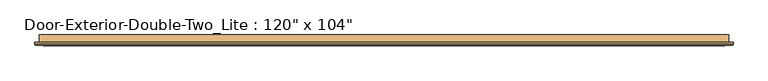
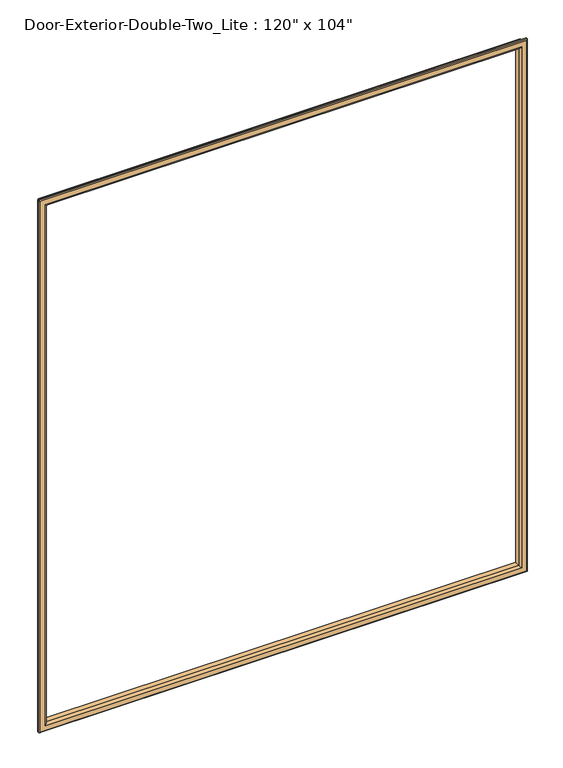
"""IFC4 building model written with IfcOpenShell, lengths in millimetres: door geometry."""

from ifc_helpers import new_model, si_unit, frame, origin, place, context, project, spatial, ellipse_curve, source, transform, mapped, element, save
from ifc_brep_helpers import plane_surface, cylinder_surface, advanced_brep


def door_2971dfc0(model_context):
    return source(origin(), model_context, "Body", "AdvancedBrep", [
        advanced_brep(
        [(-1371.6, 50.8, 1117.6), (-1371.6, 38.1, 1117.6), (-1371.6, 38.1, 2524.125), (-1371.6, 50.8, 2524.125), (-1359.6, 37.1, 1129.6), (-1359.6, 50.8, 1129.6), (-1359.6, 50.8, 2512.125), (-1359.6, 37.1, 2512.125), (-1364.6, 32.1, 1124.6), (-1364.6, 32.1, 2517.125), (-1379.6, 34.1, 1109.6), (-1377.6, 32.1, 1111.6), (-1377.6, 32.1, 2530.125), (-1379.6, 34.1, 2532.125), (-1379.6, 38.1, 1109.6), (-1379.6, 38.1, 2532.125), (-152.4, 38.1, 2524.125), (-152.4, 50.8, 2524.125), (-164.4, 50.8, 2512.125), (-164.4, 37.1, 2512.125), (-159.4, 32.1, 2517.125), (-146.4, 32.1, 2530.125), (-144.4, 34.1, 2532.125), (-144.4, 38.1, 2532.125), (-152.4, 38.1, 1117.6), (-152.4, 50.8, 1117.6), (-164.4, 50.8, 1129.6), (-164.4, 37.1, 1129.6), (-159.4, 32.1, 1124.6), (-146.4, 32.1, 1111.6), (-144.4, 34.1, 1109.6), (-144.4, 38.1, 1109.6)],
        [
            (0, 1),
            (1, 2),
            (2, 3),
            (3, 0),
            (4, 5),
            (5, 6),
            (6, 7),
            (7, 4),
            (8, 4, ellipse_curve(frame((-1364.6, 37.1, 1124.6), z_axis=(-0.7071067811865475, 0.0, 0.7071067811865475), x_axis=(-0.7071067811865474, 0.0, -0.7071067811865476)), 7.0710678, 5.0)),
            (7, 9, ellipse_curve(frame((-1364.6, 37.1, 2517.125), z_axis=(-0.7071067811865475, 0.0, -0.7071067811865475), x_axis=(0.7071067811865474, 0.0, -0.7071067811865476)), 7.0710678, 5.0)),
            (9, 8),
            (10, 11, ellipse_curve(frame((-1377.6, 34.1, 1111.6), z_axis=(-0.7071067811865475, 0.0, 0.7071067811865475), x_axis=(-0.7071067811865474, 0.0, -0.7071067811865476)), 2.8284271, 2.0)),
            (11, 12),
            (12, 13, ellipse_curve(frame((-1377.6, 34.1, 2530.125), z_axis=(-0.7071067811865475, 0.0, -0.7071067811865475), x_axis=(0.7071067811865474, 0.0, -0.7071067811865476)), 2.8284271, 2.0)),
            (13, 10),
            (14, 10),
            (13, 15),
            (15, 14),
            (2, 16),
            (16, 17),
            (17, 3),
            (6, 18),
            (18, 19),
            (19, 7),
            (19, 20, ellipse_curve(frame((-159.4, 37.1, 2517.125), z_axis=(-0.7071067811865475, 0.0, 0.7071067811865475), x_axis=(-0.7071067811865476, 0.0, -0.7071067811865474)), 7.0710678, 5.0)),
            (20, 9),
            (12, 21),
            (21, 22, ellipse_curve(frame((-146.4, 34.1, 2530.125), z_axis=(-0.7071067811865475, 0.0, 0.7071067811865475), x_axis=(-0.7071067811865476, 0.0, -0.7071067811865474)), 2.8284271, 2.0)),
            (22, 13),
            (22, 23),
            (23, 15),
            (16, 24),
            (24, 25),
            (25, 17),
            (18, 26),
            (26, 27),
            (27, 19),
            (27, 28, ellipse_curve(frame((-159.4, 37.1, 1124.6), z_axis=(0.7071067811865475, 0.0, 0.7071067811865475), x_axis=(-0.7071067811865474, 0.0, 0.7071067811865476)), 7.0710678, 5.0)),
            (28, 20),
            (21, 29),
            (29, 30, ellipse_curve(frame((-146.4, 34.1, 1111.6), z_axis=(0.7071067811865475, 0.0, 0.7071067811865475), x_axis=(-0.7071067811865474, 0.0, 0.7071067811865476)), 2.8284271, 2.0)),
            (30, 22),
            (30, 31),
            (31, 23),
            (31, 14),
            (1, 24),
            (0, 25),
            (5, 26),
            (4, 27),
            (8, 28),
            (11, 29),
            (10, 30),
        ],
        [
            plane_surface(frame((-1371.6, 38.1, 1117.6), z_axis=(-1.0, 0.0, 0.0), x_axis=(0.0, 0.0, 1.0))),
            plane_surface(frame((-1359.6, 50.8, 1129.6), z_axis=(1.0, 0.0, 0.0), x_axis=(0.0, 0.0, 1.0))),
            cylinder_surface(frame((-1364.6, 37.1, 1117.6), z_axis=(0.0, 0.0, -1.0), x_axis=(-1.0, 0.0, 0.0)), 5.0),
            cylinder_surface(frame((-1377.6, 34.1, 1117.6), z_axis=(0.0, 0.0, -1.0), x_axis=(-1.0, 0.0, 0.0)), 2.0),
            plane_surface(frame((-1379.6, 34.1, 1109.6), z_axis=(-1.0, 0.0, 0.0), x_axis=(0.0, 0.0, 1.0))),
            plane_surface(frame((-1371.6, 38.1, 2524.125), z_axis=(0.0, 0.0, 1.0), x_axis=(1.0, 0.0, 0.0))),
            plane_surface(frame((-1359.6, 50.8, 2512.125), z_axis=(0.0, 0.0, -1.0), x_axis=(1.0, 0.0, 0.0))),
            cylinder_surface(frame((-1371.6, 37.1, 2517.125), z_axis=(-1.0, 0.0, 0.0), x_axis=(0.0, 0.0, 1.0)), 5.0),
            cylinder_surface(frame((-1371.6, 34.1, 2530.125), z_axis=(-1.0, 0.0, 0.0), x_axis=(0.0, 0.0, 1.0)), 2.0),
            plane_surface(frame((-1379.6, 34.1, 2532.125), z_axis=(0.0, 0.0, 1.0), x_axis=(1.0, 0.0, 0.0))),
            plane_surface(frame((-152.4, 38.1, 2524.125), z_axis=(1.0, 0.0, 0.0), x_axis=(0.0, 0.0, -1.0))),
            plane_surface(frame((-164.4, 50.8, 2512.125), z_axis=(-1.0, 0.0, 0.0), x_axis=(0.0, 0.0, -1.0))),
            cylinder_surface(frame((-159.4, 37.1, 2524.125), z_axis=(0.0, 0.0, 1.0), x_axis=(1.0, 0.0, 0.0)), 5.0),
            cylinder_surface(frame((-146.4, 34.1, 2524.125), z_axis=(0.0, 0.0, 1.0), x_axis=(1.0, 0.0, 0.0)), 2.0),
            plane_surface(frame((-144.4, 34.1, 2532.125), z_axis=(1.0, 0.0, 0.0), x_axis=(0.0, 0.0, -1.0))),
            plane_surface(frame((-144.4, 38.1, 1109.6), z_axis=(0.0, 1.0, 0.0), x_axis=(-1.0, 0.0, 0.0))),
            plane_surface(frame((-152.4, 38.1, 1117.6), z_axis=(0.0, 0.0, -1.0), x_axis=(-1.0, 0.0, 0.0))),
            plane_surface(frame((-152.4, 50.8, 1117.6), z_axis=(0.0, 1.0, 0.0), x_axis=(-1.0, 0.0, 0.0))),
            plane_surface(frame((-164.4, 50.8, 1129.6), z_axis=(0.0, 0.0, 1.0), x_axis=(-1.0, 0.0, 0.0))),
            cylinder_surface(frame((-152.4, 37.1, 1124.6), z_axis=(1.0, 0.0, 0.0), x_axis=(0.0, 0.0, -1.0)), 5.0),
            plane_surface(frame((-159.4, 32.1, 1124.6), z_axis=(0.0, -1.0, 0.0), x_axis=(-1.0, 0.0, 0.0))),
            cylinder_surface(frame((-152.4, 34.1, 1111.6), z_axis=(1.0, 0.0, 0.0), x_axis=(0.0, 0.0, -1.0)), 2.0),
            plane_surface(frame((-144.4, 34.1, 1109.6), z_axis=(0.0, 0.0, -1.0), x_axis=(-1.0, 0.0, 0.0))),
        ],
        [
            (0, [[1, 2, 3, 4]]),
            (1, [[5, 6, 7, 8]]),
            (2, [[9, -8, 10, 11]]),
            (3, [[12, 13, 14, 15]]),
            (4, [[16, -15, 17, 18]]),
            (5, [[-3, 19, 20, 21]]),
            (6, [[-7, 22, 23, 24]]),
            (7, [[-10, -24, 25, 26]]),
            (8, [[-14, 27, 28, 29]]),
            (9, [[-17, -29, 30, 31]]),
            (10, [[-20, 32, 33, 34]]),
            (11, [[-23, 35, 36, 37]]),
            (12, [[-25, -37, 38, 39]]),
            (13, [[-28, 40, 41, 42]]),
            (14, [[-30, -42, 43, 44]]),
            (15, [[-31, -44, 45, -18], [46, -32, -19, -2]]),
            (16, [[-33, -46, -1, 47]]),
            (17, [[-21, -34, -47, -4], [48, -35, -22, -6]]),
            (18, [[-36, -48, -5, 49]]),
            (19, [[-38, -49, -9, 50]]),
            (20, [[51, -40, -27, -13], [-26, -39, -50, -11]]),
            (21, [[-41, -51, -12, 52]]),
            (22, [[-43, -52, -16, -45]]),
        ],
    ),
    ])


if __name__ == "__main__":
    model = new_model("IFC4")
    model_context = context("Model", 3, world=origin())
    ifc_project = project(units=[si_unit("LENGTHUNIT", "METRE", prefix="MILLI")], contexts=[model_context])
    site = spatial("IfcSite", under=ifc_project)
    building = spatial("IfcBuilding", under=site)
    placement = place(None, origin())
    door_shape = door_2971dfc0(model_context)
    element("IfcDoor", 1, ObjectType="Door-Exterior-Double-Two_Lite : 120\" x 104\"", at=placement, inside=building, context=model_context, shape_type="MappedRepresentation", body=[
        mapped(door_shape, transform((0.0, 0.0, 0.0), x_axis=(1.0, 0.0, 0.0), y_axis=(0.0, 1.0, 0.0), z_axis=(0.0, 0.0, 1.0))),
    ])
    save(model, "model.ifc")

# Revit data of these elements
# Type "Door-Exterior-Double-Two_Lite : 120\" x 104\""
#   Type Mark = "10"
#   Assembly Code = "B2030100"
#   Analytic Construction = "Metal frame, double glass door"
#   Top Rail = 0' - 4 5/8"
#   Threshold Length [instance default] = 10' - 4"
#   Threshold Offset [instance default] = 0' - 0 1/2"
#   Thickness = 0' - 1 3/4"
#   Thermal Resistance (R) = 1.3794 (h·ft²·°F)/BTU
#   Swing Angle [instance default] = 90.00°
#   Strike Height = 3' - 4"
#   Stiles = 0' - 6"
#   SinglePanelWidth = 5' - 0"
#   Rough Width [instance default] = 10' - 4"
#   Rough Height [instance default] = 9' - 0"
#   MFOpeningHeight [instance default] = 0' - 4"
#   MFOpeningWidth [instance default] = 0' - 4"
#   Lock Rail = 0' - 8"
#   Inset Calculate [instance default] = 0' - 4"
#   Masonry Inset [instance default] = 0' - 1"
#   Height = 8' - 8"
#   Width = 10' - 0"
#   Heat Transfer Coefficient (U) = 0.7250 BTU/(h·ft²·°F)
#   Glass Thickness = 0' - 0 3/4"
#   Masonry Frame Depth = 0' - 5 3/4"
#   Bottom Rail = 0' - 10"
#   Threshold [instance default] = yes
#   Masonry Frame [instance default] = yes
#   Function = 1
#   Dry Wall Frame [instance default] = no
#   Threshold Material = none
#   Panic Bar Material = Metal - Stainless Steel
#   Panel Material = Metal - Painted - Grey
#   Glass Stop Material = Metal - Painted - Grey
#   Frame Material = Metal - Painted - Grey
#   Exterior Pull Material = Metal - Stainless Steel
#   Visual Light Transmittance = 0
#   Solar Heat Gain Coefficient = 0
#   Wall Closure = (empty or 0)
# Element 1 (IfcDoor, "Door-Exterior-Double-Two_Lite : 120\" x 104\"")
#   Materials on its faces: "Metal - Painted - Grey", "Metal - Stainless Steel", "Glass"
# Materials
#   "Metal - Stainless Steel": class "Metal", colour RGB 247 247 247, transparency 0
#   "Metal - Painted - Grey": class "Paint", colour RGB 104 104 104, transparency 0, Cost = 0
#   "Glass": class "Glass", colour RGB 0 128 192, transparency 0.75, Description = "Soda Lime Glass", Cost = 0
